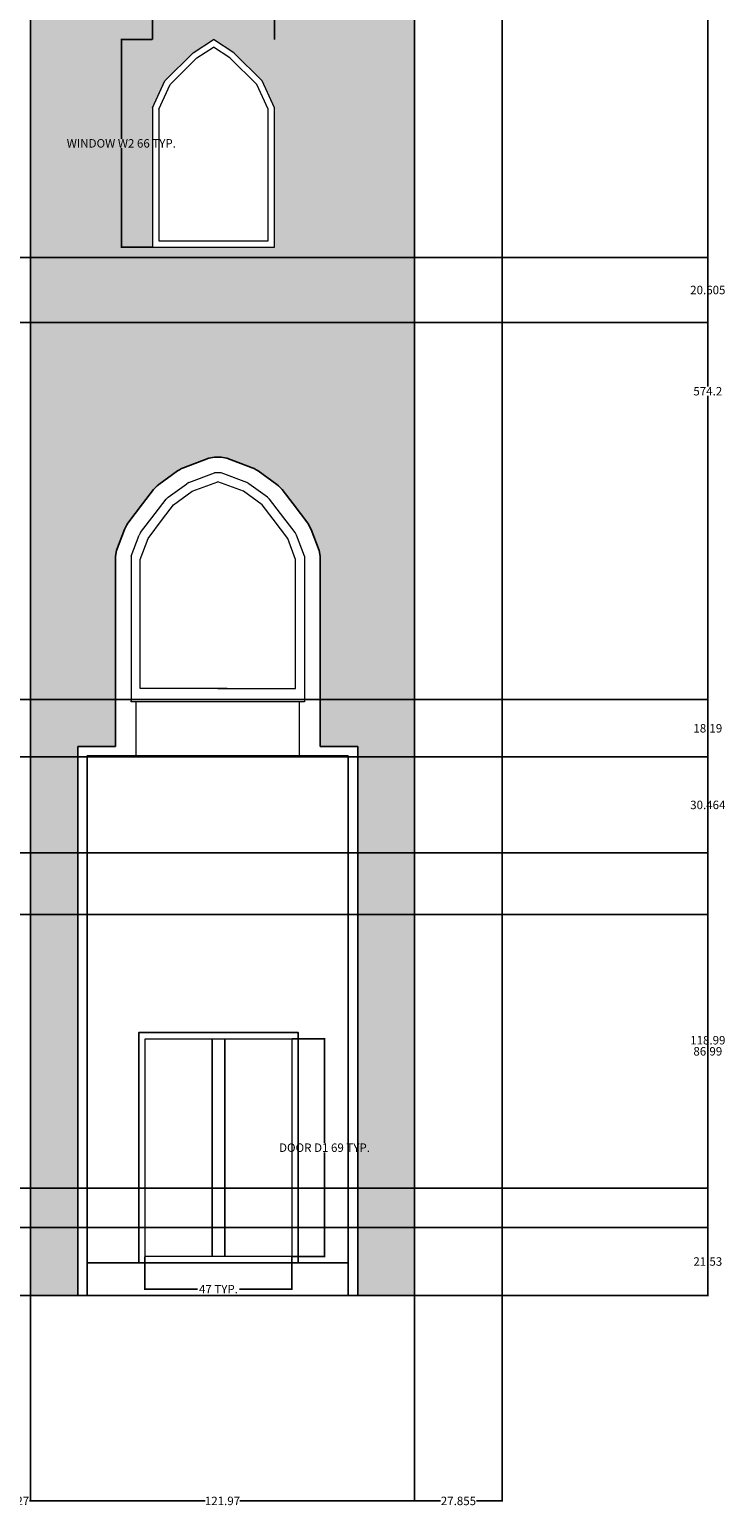
# Model space of a CAD drawing. Units: inches. Extents: x 2 to 1442, y 20 to 729.
# Tile 7 of 8: x 1221 to 1442, y 20 to 489. Entities that reach past the tile are written whole.
import ezdxf

# ---------------------------------------------------------------- set-up
doc = ezdxf.new("R2010")
doc.units = ezdxf.units.IN
doc.header["$MEASUREMENT"] = 0
for name, color, linetype, lineweight in [('A-ANNO-DIMS', 2, 'Continuous', 18), ('A-DOOR', 3, 'Continuous', 18), ('A-ELEV', 7, 'Continuous', 25), ('A-GLAZ', 4, 'Continuous', 18), ('A-WALL-PATT', 8, 'Continuous', 13)]:
    doc.layers.add(name, color=color, linetype=linetype, lineweight=lineweight)
doc.styles.get("Standard").update_dxf_attribs({"font": 'arial.ttf'})
doc.dimstyles.get("Standard").update_dxf_attribs({"dimtxt": 2.6875, "dimasz": 0.18, "dimexe": 0.18, "dimexo": 0.0625, "dimgap": 0.09, "dimtad": 0, "dimtih": 1, "dimtoh": 1, "dimdec": 4, "dimzin": 0, "dimdsep": 46, "dimlunit": 4, "dimtxsty": 'Standard', "dimcen": 0.09, "dimadec": 0, "dimazin": 0, "dimtfac": 1, "dimtdec": 4, "dimtofl": 0, "dimtmove": 0, "dimatfit": 3, "dimfxl": 1, "dimtolj": 1, "dimtzin": 0, "dimarcsym": 0})

# ---------------------------------------------------------------- blocks, each defined once
blk = doc.blocks.new('WIN-ARCH-TOWER')
for p, q in [((18.34, 86.78), (26.45, 89.83)), ((26.45, 89.83), (28.56, 89.83)), ((36.66, 86.78), (28.56, 89.83)), ((11.69, 82.12), (17.65, 86.41)), ((17.65, 86.41), (18.34, 86.78)), ((19.4, 83.98), (27.5, 87.02)), ((35.6, 83.98), (27.5, 87.02)), ((36.66, 86.78), (37.36, 86.41)), ((43.32, 82.12), (37.36, 86.41)), ((7.58, 76.95), (11.05, 81.5)), ((11.05, 81.5), (11.69, 82.12)), ((13.44, 79.69), (19.4, 83.98)), ((41.56, 79.69), (35.6, 83.98)), ((43.32, 82.12), (43.95, 81.5)), ((47.42, 76.95), (43.95, 81.5)), ((2.94, 70.87), (7.58, 76.95)), ((5.33, 69.05), (9.97, 75.13)), ((9.97, 75.13), (13.44, 79.69)), ((45.03, 75.13), (41.56, 79.69)), ((49.67, 69.05), (45.03, 75.13)), ((52.06, 70.87), (47.42, 76.95)), ((2.52, 70.11), (2.94, 70.87)), ((52.06, 70.87), (52.48, 70.11)), ((0, 63.44), (2.52, 70.11)), ((2.81, 62.38), (5.33, 69.05)), ((52.2, 62.38), (49.67, 69.05)), ((55, 63.44), (52.48, 70.11)), ((0, 63.44), (0, 62.38)), ((0, 62.38), (0, 17.18)), ((2.81, 21.32), (2.81, 62.38)), ((52.2, 21.32), (52.2, 62.38)), ((55, 63.44), (55, 62.38)), ((55, 62.38), (55, 17.41)), ((27.5, 21.32), (2.81, 21.32)), ((24.55, 21.32), (49.24, 21.32)), ((49.24, 21.32), (52.2, 21.32)), ((0, 17.18), (1.6, 17.18)), ((1.6, 0), (1.6, 17.18)), ((1.6, 17.18), (53.4, 17.18)), ((53.4, 0), (53.4, 17.18)), ((53.4, 17.18), (55.01, 17.18)), ((55.01, 17.18), (55, 17.41))]:
    blk.add_line(p, q)
blk = doc.blocks.new('WIN-ARCH-SMALL')
for points in [[(0, 44.18), (3.93, 52.78), (12.87, 61.71), (19.37, 65.87)], [(38.74, 44.18), (34.82, 52.78), (25.87, 61.71), (19.37, 65.87)], [(2, 43.74), (5.6, 51.62), (14.13, 60.14), (19.37, 63.49)], [(36.74, 43.74), (33.15, 51.62), (24.61, 60.14), (19.37, 63.49)], [(0, 44.18), (0, 0), (38.74, 0), (38.74, 44.18)], [(2, 43.74), (2, 2), (36.74, 2), (36.74, 43.74)]]:
    blk.add_lwpolyline(points)
blk = doc.blocks.new('DOOR-DOUBLE')
for points in [[(23.31, 0), (0, 0), (0, 69.12), (23.31, 69.12)], [(23.31, 69.12), (46.63, 69.12), (46.63, 0), (23.31, 0)]]:
    blk.add_lwpolyline(points)
blk = doc.blocks.new('*D7')
at = {"layer": 'A-ANNO-DIMS', "color": 0, "lineweight": -2, "transparency": 16777216}
for p, q in [((1259.99, 486.02), (1249.99, 486.02)), ((1250.17, 485.84), (1250.17, 454.56)), ((1250.17, 420.33), (1250.17, 451.6)), ((1259.99, 420.15), (1249.99, 420.15))]:
    blk.add_line(p, q, dxfattribs=at)
at = {"layer": 'A-ANNO-DIMS', "color": 0, "transparency": 16777216}
for points in [[(1250.14, 485.84), (1250.2, 485.84), (1250.17, 486.02)], [(1250.14, 420.33), (1250.2, 420.33), (1250.17, 420.15)]]:
    blk.add_solid(points, dxfattribs=at)
at = {"layer": 'Defpoints', "color": 0, "transparency": 16777216}
for p in [(1250.17, 486.02), (1260.05, 486.02), (1260.05, 420.15)]:
    blk.add_point(p, dxfattribs=at)
at = {"layer": 'A-ANNO-DIMS', "color": 0, "transparency": 16777216, "insert": (1250.17, 453.08), "char_height": 2.6875, "attachment_point": 5}
blk.add_mtext('\\A1;WINDOW W2 66 TYP.', dxfattribs=at)
blk = doc.blocks.new('*D8')
at = {"layer": 'A-ANNO-DIMS', "color": 0, "lineweight": -2, "transparency": 16777216}
for p, q in [((1260.05, 486.08), (1260.05, 496.08)), ((1260.23, 495.9), (1272.79, 495.9)), ((1298.61, 495.9), (1286.05, 495.9)), ((1298.79, 486.08), (1298.79, 496.08))]:
    blk.add_line(p, q, dxfattribs=at)
at = {"layer": 'A-ANNO-DIMS', "color": 0, "transparency": 16777216}
for points in [[(1260.23, 495.93), (1260.23, 495.87), (1260.05, 495.9)], [(1298.61, 495.93), (1298.61, 495.87), (1298.79, 495.9)]]:
    blk.add_solid(points, dxfattribs=at)
at = {"layer": 'Defpoints', "color": 0, "transparency": 16777216}
for p in [(1298.79, 495.9), (1260.05, 486.02), (1298.79, 486.02)]:
    blk.add_point(p, dxfattribs=at)
at = {"layer": 'A-ANNO-DIMS', "color": 0, "transparency": 16777216, "insert": (1279.42, 495.9), "char_height": 2.6875, "attachment_point": 5}
blk.add_mtext('\\A1;39 TYP.', dxfattribs=at)
blk = doc.blocks.new('*D11')
at = {"layer": 'A-ANNO-DIMS', "color": 0, "lineweight": -2, "transparency": 16777216}
for p, q in [((1304.37, 168.74), (1314.86, 168.74)), ((1314.68, 168.56), (1314.68, 135.66)), ((1314.68, 99.8), (1314.68, 132.7)), ((1304.37, 99.62), (1314.86, 99.62))]:
    blk.add_line(p, q, dxfattribs=at)
at = {"layer": 'A-ANNO-DIMS', "color": 0, "transparency": 16777216}
for points in [[(1314.65, 168.56), (1314.71, 168.56), (1314.68, 168.74)], [(1314.65, 99.8), (1314.71, 99.8), (1314.68, 99.62)]]:
    blk.add_solid(points, dxfattribs=at)
at = {"layer": 'Defpoints', "color": 0, "transparency": 16777216}
for p in [(1304.31, 168.74), (1314.68, 168.74), (1304.31, 99.62)]:
    blk.add_point(p, dxfattribs=at)
at = {"layer": 'A-ANNO-DIMS', "color": 0, "transparency": 16777216, "insert": (1314.68, 134.18), "char_height": 2.6875, "attachment_point": 5}
blk.add_mtext('\\A1;DOOR D1 69 TYP.', dxfattribs=at)
blk = doc.blocks.new('*D12')
at = {"layer": 'A-ANNO-DIMS', "color": 0, "lineweight": -2, "transparency": 16777216}
for p, q in [((1257.68, 99.56), (1257.68, 89.07)), ((1304.31, 99.56), (1304.31, 89.07)), ((1257.86, 89.25), (1274.31, 89.25)), ((1304.13, 89.25), (1287.68, 89.25))]:
    blk.add_line(p, q, dxfattribs=at)
at = {"layer": 'A-ANNO-DIMS', "color": 0, "transparency": 16777216}
for points in [[(1257.86, 89.28), (1257.86, 89.22), (1257.68, 89.25)], [(1304.13, 89.28), (1304.13, 89.22), (1304.31, 89.25)]]:
    blk.add_solid(points, dxfattribs=at)
at = {"layer": 'Defpoints', "color": 0, "transparency": 16777216}
for p in [(1257.68, 99.62), (1304.31, 99.62), (1304.31, 89.25)]:
    blk.add_point(p, dxfattribs=at)
at = {"layer": 'A-ANNO-DIMS', "color": 0, "transparency": 16777216, "insert": (1281, 89.25), "char_height": 2.6875, "attachment_point": 5}
blk.add_mtext('\\A1;47 TYP.', dxfattribs=at)
blk = doc.blocks.new('*D28')
at = {"layer": 'A-ANNO-DIMS', "color": 0, "lineweight": -2, "transparency": 16777216}
for p, q in [((1211.37, 87.21), (1211.37, 21.84)), ((1221.3, 87.21), (1221.3, 21.84)), ((1211.55, 22.02), (1211.71, 22.02)), ((1221.12, 22.02), (1220.96, 22.02))]:
    blk.add_line(p, q, dxfattribs=at)
at = {"layer": 'A-ANNO-DIMS', "color": 0, "transparency": 16777216}
for points in [[(1211.55, 22.05), (1211.55, 21.99), (1211.37, 22.02)], [(1221.12, 22.05), (1221.12, 21.99), (1221.3, 22.02)]]:
    blk.add_solid(points, dxfattribs=at)
at = {"layer": 'Defpoints', "color": 0, "transparency": 16777216}
for p in [(1211.37, 87.27), (1221.3, 87.27), (1221.3, 22.02)]:
    blk.add_point(p, dxfattribs=at)
at = {"layer": 'A-ANNO-DIMS', "color": 0, "transparency": 16777216, "insert": (1216.33, 22.02), "char_height": 2.688, "attachment_point": 5}
blk.add_mtext('\\A1;9.927', dxfattribs=at)
blk = doc.blocks.new('*D29')
at = {"layer": 'A-ANNO-DIMS', "color": 0, "lineweight": -2, "transparency": 16777216}
for p, q in [((1221.3, 87.21), (1221.3, 21.84)), ((1343.27, 87.21), (1343.27, 21.84)), ((1221.48, 22.02), (1276.74, 22.02)), ((1343.09, 22.02), (1287.82, 22.02))]:
    blk.add_line(p, q, dxfattribs=at)
at = {"layer": 'A-ANNO-DIMS', "color": 0, "transparency": 16777216}
for points in [[(1221.48, 22.05), (1221.48, 21.99), (1221.3, 22.02)], [(1343.09, 22.05), (1343.09, 21.99), (1343.27, 22.02)]]:
    blk.add_solid(points, dxfattribs=at)
at = {"layer": 'Defpoints', "color": 0, "transparency": 16777216}
for p in [(1221.3, 87.27), (1343.27, 87.27), (1343.27, 22.02)]:
    blk.add_point(p, dxfattribs=at)
at = {"layer": 'A-ANNO-DIMS', "color": 0, "transparency": 16777216, "insert": (1282.28, 22.02), "char_height": 2.688, "attachment_point": 5}
blk.add_mtext('\\A1;121.97', dxfattribs=at)
blk = doc.blocks.new('*D30')
at = {"layer": 'A-ANNO-DIMS', "color": 0, "lineweight": -2, "transparency": 16777216}
for p, q in [((1343.27, 87.21), (1343.27, 21.84)), ((1371.12, 87.21), (1371.12, 21.84)), ((1343.45, 22.02), (1351.5, 22.02)), ((1370.94, 22.02), (1362.9, 22.02))]:
    blk.add_line(p, q, dxfattribs=at)
at = {"layer": 'A-ANNO-DIMS', "color": 0, "transparency": 16777216}
for points in [[(1343.45, 22.05), (1343.45, 21.99), (1343.27, 22.02)], [(1370.94, 22.05), (1370.94, 21.99), (1371.12, 22.02)]]:
    blk.add_solid(points, dxfattribs=at)
at = {"layer": 'Defpoints', "color": 0, "transparency": 16777216}
for p in [(1343.27, 87.27), (1371.12, 87.27), (1371.12, 22.02)]:
    blk.add_point(p, dxfattribs=at)
at = {"layer": 'A-ANNO-DIMS', "color": 0, "transparency": 16777216, "insert": (1357.2, 22.02), "char_height": 2.688, "attachment_point": 5}
blk.add_mtext('\\A1;27.855', dxfattribs=at)
blk = doc.blocks.new('*D33')
at = {"layer": 'A-ANNO-DIMS', "color": 0, "lineweight": -2, "transparency": 16777216}
for p, q in [((722.06, 661.5), (1436.55, 661.5)), ((1436.37, 661.32), (1436.37, 375.85)), ((1436.37, 87.45), (1436.37, 372.92)), ((1371.19, 87.27), (1436.55, 87.27))]:
    blk.add_line(p, q, dxfattribs=at)
at = {"layer": 'A-ANNO-DIMS', "color": 0, "transparency": 16777216}
for points in [[(1436.34, 661.32), (1436.4, 661.32), (1436.37, 661.5)], [(1436.34, 87.45), (1436.4, 87.45), (1436.37, 87.27)]]:
    blk.add_solid(points, dxfattribs=at)
at = {"layer": 'Defpoints', "color": 0, "transparency": 16777216}
for p in [(722, 661.5), (1436.37, 661.5), (1371.12, 87.27)]:
    blk.add_point(p, dxfattribs=at)
at = {"layer": 'A-ANNO-DIMS', "color": 0, "transparency": 16777216, "insert": (1436.37, 374.39), "char_height": 2.688, "attachment_point": 5}
blk.add_mtext('\\A1;574.2', dxfattribs=at)
blk = doc.blocks.new('*D50')
at = {"layer": 'A-ANNO-DIMS', "color": 0, "lineweight": -2, "transparency": 16777216}
for p, q in [((433.03, 108.8), (1436.55, 108.8)), ((1436.37, 108.62), (1436.37, 99.5)), ((1436.37, 87.45), (1436.37, 96.57)), ((433.03, 87.27), (1436.55, 87.27))]:
    blk.add_line(p, q, dxfattribs=at)
at = {"layer": 'A-ANNO-DIMS', "color": 0, "transparency": 16777216}
for points in [[(1436.34, 108.62), (1436.4, 108.62), (1436.37, 108.8)], [(1436.34, 87.45), (1436.4, 87.45), (1436.37, 87.27)]]:
    blk.add_solid(points, dxfattribs=at)
at = {"layer": 'Defpoints', "color": 0, "transparency": 16777216}
for p in [(432.97, 108.8), (1436.37, 108.8), (432.97, 87.27)]:
    blk.add_point(p, dxfattribs=at)
at = {"layer": 'A-ANNO-DIMS', "color": 0, "transparency": 16777216, "insert": (1436.37, 98.04), "char_height": 2.688, "attachment_point": 5}
blk.add_mtext('\\A1;21.53', dxfattribs=at)
blk = doc.blocks.new('*D51')
at = {"layer": 'A-ANNO-DIMS', "color": 0, "lineweight": -2, "transparency": 16777216}
for p, q in [((426.83, 227.79), (1436.55, 227.79)), ((1436.37, 227.61), (1436.37, 169.76)), ((1436.37, 108.98), (1436.37, 166.83)), ((433.03, 108.8), (1436.55, 108.8))]:
    blk.add_line(p, q, dxfattribs=at)
at = {"layer": 'A-ANNO-DIMS', "color": 0, "transparency": 16777216}
for points in [[(1436.34, 227.61), (1436.4, 227.61), (1436.37, 227.79)], [(1436.34, 108.98), (1436.4, 108.98), (1436.37, 108.8)]]:
    blk.add_solid(points, dxfattribs=at)
at = {"layer": 'Defpoints', "color": 0, "transparency": 16777216}
for p in [(426.77, 227.79), (1436.37, 227.79), (432.97, 108.8)]:
    blk.add_point(p, dxfattribs=at)
at = {"layer": 'A-ANNO-DIMS', "color": 0, "transparency": 16777216, "insert": (1436.37, 168.3), "char_height": 2.688, "attachment_point": 5}
blk.add_mtext('\\A1;118.99', dxfattribs=at)
blk = doc.blocks.new('*D52')
at = {"layer": 'A-ANNO-DIMS', "color": 0, "lineweight": -2, "transparency": 16777216}
for p, q in [((433.03, 258.25), (1436.55, 258.25)), ((1436.37, 258.07), (1436.37, 244.49)), ((1436.37, 227.97), (1436.37, 241.56)), ((426.83, 227.79), (1436.55, 227.79))]:
    blk.add_line(p, q, dxfattribs=at)
at = {"layer": 'A-ANNO-DIMS', "color": 0, "transparency": 16777216}
for points in [[(1436.34, 258.07), (1436.4, 258.07), (1436.37, 258.25)], [(1436.34, 227.97), (1436.4, 227.97), (1436.37, 227.79)]]:
    blk.add_solid(points, dxfattribs=at)
at = {"layer": 'Defpoints', "color": 0, "transparency": 16777216}
for p in [(432.97, 258.25), (1436.37, 258.25), (426.77, 227.79)]:
    blk.add_point(p, dxfattribs=at)
at = {"layer": 'A-ANNO-DIMS', "color": 0, "transparency": 16777216, "insert": (1436.37, 243.02), "char_height": 2.688, "attachment_point": 5}
blk.add_mtext('\\A1;30.464', dxfattribs=at)
blk = doc.blocks.new('*D53')
at = {"layer": 'A-ANNO-DIMS', "color": 0, "lineweight": -2, "transparency": 16777216}
for p, q in [((433.03, 276.44), (1436.55, 276.44)), ((1436.37, 276.26), (1436.37, 268.81)), ((1436.37, 258.43), (1436.37, 265.89)), ((433.03, 258.25), (1436.55, 258.25))]:
    blk.add_line(p, q, dxfattribs=at)
at = {"layer": 'A-ANNO-DIMS', "color": 0, "transparency": 16777216}
for points in [[(1436.34, 276.26), (1436.4, 276.26), (1436.37, 276.44)], [(1436.34, 258.43), (1436.4, 258.43), (1436.37, 258.25)]]:
    blk.add_solid(points, dxfattribs=at)
at = {"layer": 'Defpoints', "color": 0, "transparency": 16777216}
for p in [(432.97, 276.44), (1436.37, 276.44), (432.97, 258.25)]:
    blk.add_point(p, dxfattribs=at)
at = {"layer": 'A-ANNO-DIMS', "color": 0, "transparency": 16777216, "insert": (1436.37, 267.35), "char_height": 2.688, "attachment_point": 5}
blk.add_mtext('\\A1;18.19', dxfattribs=at)
blk = doc.blocks.new('*D55')
at = {"layer": 'A-ANNO-DIMS', "color": 0, "lineweight": -2, "transparency": 16777216}
for p, q in [((391.01, 416.82), (1436.55, 416.82)), ((1436.37, 416.64), (1436.37, 407.98)), ((1436.37, 396.4), (1436.37, 405.06)), ((394.77, 396.22), (1436.55, 396.22))]:
    blk.add_line(p, q, dxfattribs=at)
at = {"layer": 'A-ANNO-DIMS', "color": 0, "transparency": 16777216}
for points in [[(1436.34, 416.64), (1436.4, 416.64), (1436.37, 416.82)], [(1436.34, 396.4), (1436.4, 396.4), (1436.37, 396.22)]]:
    blk.add_solid(points, dxfattribs=at)
at = {"layer": 'Defpoints', "color": 0, "transparency": 16777216}
for p in [(390.95, 416.82), (1436.37, 416.82), (394.7, 396.22)]:
    blk.add_point(p, dxfattribs=at)
at = {"layer": 'A-ANNO-DIMS', "color": 0, "transparency": 16777216, "insert": (1436.37, 406.52), "char_height": 2.688, "attachment_point": 5}
blk.add_mtext('\\A1;20.605', dxfattribs=at)
blk = doc.blocks.new('*D60')
at = {"layer": 'A-ANNO-DIMS', "color": 0, "lineweight": -2, "transparency": 16777216}
for p, q in [((414.48, 208.27), (1436.55, 208.27)), ((1436.37, 208.09), (1436.37, 166.24)), ((1436.37, 121.46), (1436.37, 163.32)), ((414.48, 121.28), (1436.55, 121.28))]:
    blk.add_line(p, q, dxfattribs=at)
at = {"layer": 'A-ANNO-DIMS', "color": 0, "transparency": 16777216}
for points in [[(1436.34, 208.09), (1436.4, 208.09), (1436.37, 208.27)], [(1436.34, 121.46), (1436.4, 121.46), (1436.37, 121.28)]]:
    blk.add_solid(points, dxfattribs=at)
at = {"layer": 'Defpoints', "color": 0, "transparency": 16777216}
for p in [(414.42, 208.27), (1436.37, 208.27), (414.42, 121.28)]:
    blk.add_point(p, dxfattribs=at)
at = {"layer": 'A-ANNO-DIMS', "color": 0, "transparency": 16777216, "insert": (1436.37, 164.78), "char_height": 2.688, "attachment_point": 5}
blk.add_mtext('\\A1;86.99', dxfattribs=at)

msp = doc.modelspace()

# ---------------------------------------------------------------- hatches: boundary and pattern name
at = {"layer": 'A-WALL-PATT'}
h = msp.add_hatch(dxfattribs=at)
h.set_pattern_fill('BRASS', color=256, scale=14)
h.paths.add_polyline_path([(1221.296, 494.0357), (1343.2694, 494.0357), (1343.2694, 87.2714), (1325.228, 87.2714), (1325.228, 261.6116), (1313.3063, 261.6116), (1313.3063, 275.7919), (1313.3063, 320.992), (1313.3063, 322.0535), (1312.9828, 323.8227), (1310.4604, 330.4901), (1309.3395, 332.5101), (1304.6979, 338.5974), (1301.0035, 343.4423), (1299.8408, 344.5736), (1293.3137, 349.2734), (1292.0313, 349.9601), (1283.618, 353.1203), (1281.8598, 353.4396), (1279.7501, 353.4396), (1277.992, 353.1203), (1269.5786, 349.9601), (1268.2962, 349.2734), (1261.7691, 344.5736), (1260.6064, 343.4423), (1256.912, 338.5974), (1252.0504, 332.2216), (1251.278, 330.8295), (1248.6271, 323.8227), (1248.3037, 322.0535), (1248.3037, 320.992), (1248.3037, 276.0187), (1248.3037, 261.5562), (1236.3716, 261.5562), (1236.3716, 87.2714), (1221.296, 87.2714)])
h.paths.add_polyline_path([(1298.7943, 420.1495), (1298.7943, 464.3282), (1294.8674, 472.9254), (1285.9225, 481.8631), (1279.4227, 486.0178), (1272.9229, 481.8631), (1263.978, 472.9254), (1260.0512, 464.3282), (1260.0512, 420.1495)], flags=16)
h.paths.add_polyline_path([(1296.7943, 422.1495), (1296.7943, 463.893), (1293.1982, 471.7659), (1284.6625, 480.2948), (1279.4227, 483.6441), (1274.183, 480.2948), (1265.6472, 471.7659), (1262.0512, 463.893), (1262.0512, 422.1495)], flags=0)

# ---------------------------------------------------------------- linework, layer by layer
at = {"layer": 'A-ELEV'}
for p, q in [((1371.1242, 520.5823), (1371.1242, 464.6214)), ((1371.1242, 423.2714), (1371.1242, 471.2714)), ((1371.1242, 255.2714), (1371.1242, 423.2714)), ((1269.8889, 350.0767), (1277.992, 353.1203)), ((1281.8598, 353.4396), (1279.7501, 353.4396)), ((1291.7211, 350.0767), (1283.618, 353.1203)), ((1262.0692, 344.7897), (1268.0273, 349.0797)), ((1269.2865, 349.8037), (1268.5884, 349.4298)), ((1293.0215, 349.4298), (1292.3234, 349.8037)), ((1299.5407, 344.7897), (1293.5826, 349.0797)), ((1256.912, 338.5974), (1260.3822, 343.1483)), ((1261.5041, 344.3157), (1260.8714, 343.7002)), ((1300.7385, 343.7002), (1300.1059, 344.3157)), ((1304.6979, 338.5974), (1301.2277, 343.1483)), ((1252.2704, 332.5101), (1256.912, 338.5974)), ((1309.3395, 332.5101), (1304.6979, 338.5974)), ((1248.6271, 323.8227), (1251.1496, 330.4901)), ((1251.8743, 331.9043), (1251.454, 331.1468)), ((1312.9828, 323.8227), (1310.4604, 330.4901)), ((1248.3037, 322.0535), (1248.3037, 320.992)), ((1248.3037, 320.992), (1248.3037, 276.0187)), ((1313.3063, 322.0535), (1313.3063, 320.992)), ((1313.3063, 320.992), (1313.3063, 275.7919)), ((1248.3037, 276.0187), (1248.3037, 261.5562)), ((1313.3063, 275.7919), (1313.3063, 261.6116)), ((1236.3716, 87.2714), (1236.3716, 261.5562)), ((1236.3716, 261.5562), (1248.3037, 261.5562)), ((1325.228, 261.6116), (1313.3063, 261.6116)), ((1325.228, 87.2714), (1325.228, 261.6116)), ((1325.228, 258.6116), (1325.228, 258.6116)), ((1371.1242, 87.2714), (1371.1242, 255.2714)), ((1322.228, 227.7901), (1239.3716, 227.7901)), ((1322.228, 97.6222), (1239.3716, 97.6222)), ((721.8257, 87.2714), (1371.1242, 87.2714))]:
    msp.add_line(p, q, dxfattribs=at)
for points in [[(1343.2694, 494.0357), (1221.296, 494.0357), (1221.296, 87.2714), (1343.2694, 87.2714)], [(1322.228, 258.6116), (1239.3716, 258.6116), (1239.3716, 87.2714), (1322.228, 87.2714)]]:
    msp.add_lwpolyline(points, close=True, dxfattribs=at)
for points in [[(1279.7501, 353.4396), (1277.992, 353.1203)], [(1283.618, 353.1203), (1281.8598, 353.4396)], [(1268.5884, 349.4298), (1268.0273, 349.0797)], [(1269.8889, 350.0767), (1269.2865, 349.8037)], [(1292.3234, 349.8037), (1291.7211, 350.0767)], [(1293.5826, 349.0797), (1293.0215, 349.4298)], [(1260.8714, 343.7002), (1260.3822, 343.1483)], [(1262.0692, 344.7897), (1261.5041, 344.3157)], [(1300.1059, 344.3157), (1299.5407, 344.7897)], [(1301.2277, 343.1483), (1300.7385, 343.7002)], [(1251.454, 331.1468), (1251.1496, 330.4901)], [(1252.2704, 332.5101), (1251.8743, 331.9043)], [(1310.4604, 330.4901), (1309.3395, 332.5101)], [(1248.6271, 323.8227), (1248.3037, 322.0535)], [(1313.3063, 322.0535), (1312.9828, 323.8227)], [(1282.9959, 170.7392), (1255.6816, 170.7392), (1255.6816, 97.6222), (1282.9959, 97.6222)], [(1278.9959, 97.6222), (1278.9959, 97.6222), (1306.3102, 97.6222), (1306.3102, 170.7392), (1278.9959, 170.7392)], [(1278.9959, 168.7392), (1278.9959, 99.6222)], [(1282.9959, 99.6222), (1282.9959, 168.7392)]]:
    msp.add_lwpolyline(points, dxfattribs=at)

# ---------------------------------------------------------------- block references
at = {"layer": 'A-DOOR'}
msp.add_blockref('DOOR-DOUBLE', (1257.6814, 99.622), dxfattribs=at)
at = {"layer": 'A-GLAZ'}
msp.add_blockref('WIN-ARCH-SMALL', (1260.051, 420.15), dxfattribs=at)
at = {"layer": 'A-GLAZ', "extrusion": (0, 0, -1), "zscale": -1}
msp.add_blockref('WIN-ARCH-TOWER', (-1308.3064, 258.612), dxfattribs=at)

# ---------------------------------------------------------------- dimensions: what is measured, and where the dimension line sits
at = {"layer": 'A-ANNO-DIMS'}
for base, p1, p2, override, picture, middle in [((1436.3742, 661.5), (1371.1242, 87.2714), (722, 661.5), {"dimdec": 1, "dimlfac": 1, "dimrnd": 0, "dimzin": 0, "dimdsep": 46, "dimlunit": 2}, '*D33', (1436.3742, 374.3857)), ((1436.3742, 416.8211), (394.7029, 396.2159), (390.9514, 416.8211), {"dimdec": 3, "dimlfac": 1, "dimrnd": 0, "dimzin": 0, "dimdsep": 46, "dimlunit": 2}, '*D55', (1436.3742, 406.5185)), ((1436.3742, 276.443), (432.9658, 258.2539), (432.9658, 276.443), {"dimdec": 2, "dimlfac": 1, "dimrnd": 0, "dimzin": 0, "dimdsep": 46, "dimlunit": 2}, '*D53', (1436.3742, 267.3485)), ((1436.3742, 258.2539), (426.7688, 227.7901), (432.9658, 258.2539), {"dimdec": 3, "dimlfac": 1, "dimrnd": 0, "dimzin": 0, "dimdsep": 46, "dimlunit": 2}, '*D52', (1436.3742, 243.022)), ((1436.3742, 227.7901), (432.9658, 108.8033), (426.7688, 227.7901), {"dimdec": 2, "dimlfac": 1, "dimrnd": 0, "dimzin": 0, "dimdsep": 46, "dimlunit": 2}, '*D51', (1436.3742, 168.2967)), ((1436.3742, 208.2722), (414.4218, 121.2842), (414.4218, 208.2722), {"dimdec": 2, "dimlfac": 1, "dimrnd": 0, "dimzin": 0, "dimdsep": 46, "dimlunit": 2}, '*D60', (1436.3742, 164.7782)), ((1436.3742, 108.8033), (432.9658, 87.2714), (432.9658, 108.8033), {"dimdec": 2, "dimlfac": 1, "dimrnd": 0, "dimzin": 0, "dimdsep": 46, "dimlunit": 2}, '*D50', (1436.3742, 98.0373))]:
    dim = msp.add_linear_dim(base=base, p1=p1, p2=p2, angle=90, dimstyle='Standard', override=override, dxfattribs=at)
    dim.commit()
    dim.dimension.update_dxf_attribs({"geometry": picture, "text_midpoint": middle})
for base, p1, p2, picture, middle in [((1298.7943, 495.898), (1260.0512, 486.0178), (1298.7943, 486.0178), '*D8', (1279.4227, 495.898)), ((1304.3102, 89.2547), (1257.6816, 99.6222), (1304.3102, 99.6222), '*D12', (1280.9959, 89.2547))]:
    dim = msp.add_linear_dim(base=base, p1=p1, p2=p2, text='<> TYP.', dimstyle='Standard', override={"dimdec": 0, "dimrnd": 0, "dimzin": 0, "dimlunit": 2}, dxfattribs=at)
    dim.commit()
    dim.dimension.update_dxf_attribs({"geometry": picture, "text_midpoint": middle})
for base, p1, p2, text, picture, middle in [((1250.1709, 486.0178), (1260.0512, 420.1495), (1260.0512, 486.0178), 'WINDOW W2 <> TYP.', '*D7', (1250.1709, 453.0836)), ((1314.6777, 168.7392), (1304.3102, 99.6222), (1304.3102, 168.7392), 'DOOR D1 <> TYP.', '*D11', (1314.6777, 134.1807))]:
    dim = msp.add_linear_dim(base=base, p1=p1, p2=p2, angle=90, text=text, dimstyle='Standard', override={"dimdec": 0, "dimrnd": 0, "dimzin": 0, "dimlunit": 2}, dxfattribs=at)
    dim.commit()
    dim.dimension.update_dxf_attribs({"geometry": picture, "text_midpoint": middle})
for base, p1, p2, override, picture, middle in [((1221.296, 22.0214), (1211.369, 87.2714), (1221.296, 87.2714), {"dimdec": 3, "dimlfac": 1, "dimrnd": 0, "dimzin": 0, "dimdsep": 46, "dimlunit": 2}, '*D28', (1216.3325, 22.0214)), ((1343.2694, 22.0214), (1221.296, 87.2714), (1343.2694, 87.2714), {"dimdec": 2, "dimlfac": 1, "dimrnd": 0, "dimzin": 0, "dimdsep": 46, "dimlunit": 2}, '*D29', (1282.2827, 22.0214)), ((1371.1242, 22.0214), (1343.2694, 87.2714), (1371.1242, 87.2714), {"dimdec": 3, "dimlfac": 1, "dimrnd": 0, "dimzin": 0, "dimdsep": 46, "dimlunit": 2}, '*D30', (1357.1968, 22.0214))]:
    dim = msp.add_linear_dim(base=base, p1=p1, p2=p2, dimstyle='Standard', override=override, dxfattribs=at)
    dim.commit()
    dim.dimension.update_dxf_attribs({"geometry": picture, "text_midpoint": middle})

doc.saveas('drawing.dxf')
